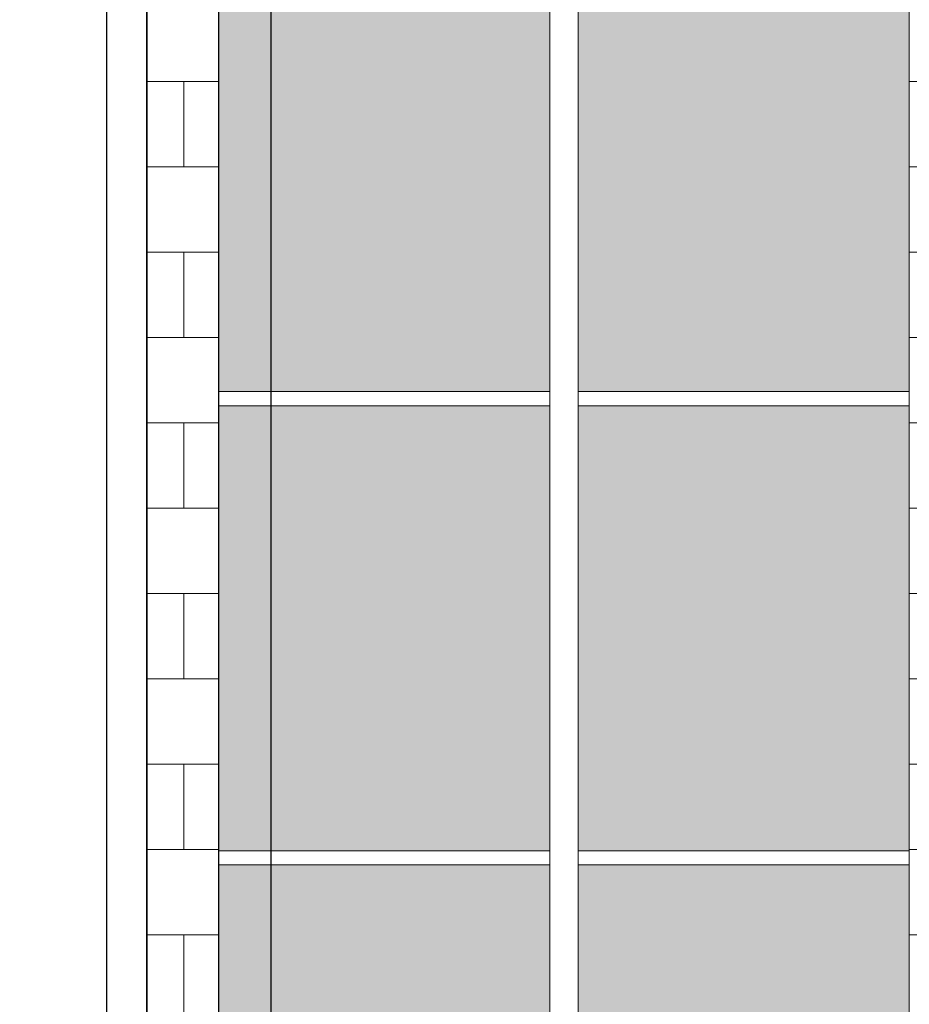
# Model space of a CAD drawing. Units: inches. Extents: x -26 to 776, y -22 to 650.
# Tile 20 of 62: x 222 to 285, y 223 to 292. Entities that reach past the tile are written whole.
import ezdxf

# ---------------------------------------------------------------- set-up
doc = ezdxf.new("R2010")
doc.units = ezdxf.units.IN
doc.header["$MEASUREMENT"] = 0
for name, color, linetype, lineweight in [('A-ANNO-DIMS', 2, 'Continuous', 18), ('A-GLAZ', 4, 'Continuous', 18), ('A-GLAZ-PATT', 9, 'Continuous', 13), ('A-WALL', 7, 'Continuous', 35), ('A-WALL-PATT', 8, 'Continuous', 13), ('A-WALL-TRIM', 7, 'Continuous', 18)]:
    doc.layers.add(name, color=color, linetype=linetype, lineweight=lineweight)
doc.styles.get("Standard").update_dxf_attribs({"font": 'arial.ttf'})
doc.dimstyles.get("Standard").update_dxf_attribs({"dimtxt": 0.5625, "dimasz": 0.18, "dimexe": 0.18, "dimexo": 0.0625, "dimgap": 0.09, "dimtad": 0, "dimtih": 1, "dimtoh": 1, "dimdec": 4, "dimzin": 0, "dimdsep": 46, "dimlunit": 4, "dimtxsty": 'Standard', "dimcen": 0.09, "dimadec": 0, "dimazin": 0, "dimtfac": 1, "dimtdec": 4, "dimtofl": 0, "dimtmove": 0, "dimatfit": 3, "dimfxl": 1, "dimtolj": 1, "dimtzin": 0, "dimarcsym": 0})

# ---------------------------------------------------------------- blocks, each defined once
blk = doc.blocks.new('WIN-ELEV-2X4-HEAD')
for p, q in [((23.276, 0), (23.276, 123)), ((25.276, 0), (25.276, 123)), ((0, 94.772), (23.276, 94.772)), ((25.276, 94.772), (48.553, 94.772)), ((0, 93.772), (23.276, 93.772)), ((25.276, 93.772), (48.553, 93.772)), ((0, 62.5), (23.276, 62.5)), ((25.276, 62.5), (48.553, 62.5)), ((0, 61.5), (23.276, 61.5)), ((25.276, 61.5), (48.553, 61.5))]:
    blk.add_line(p, q)
blk.add_lwpolyline([(48.553, 0), (0, 0), (0, 123), (48.553, 123)], close=True)
blk = doc.blocks.new('*D34')
at = {"layer": 'A-ANNO-DIMS', "color": 0, "lineweight": -2, "transparency": 16777216}
for p, q in [((228.573, 528.296), (228.573, -21.315)), ((357.303, 528.361), (357.303, -21.315)), ((228.753, -21.135), (291.707, -21.135)), ((357.123, -21.135), (294.17, -21.135))]:
    blk.add_line(p, q, dxfattribs=at)
at = {"layer": 'A-ANNO-DIMS', "color": 0, "transparency": 16777216}
for points in [[(228.753, -21.105), (228.753, -21.165), (228.573, -21.135)], [(357.123, -21.105), (357.123, -21.165), (357.303, -21.135)]]:
    blk.add_solid(points, dxfattribs=at)
at = {"layer": 'Defpoints', "color": 0, "transparency": 16777216}
for p in [(228.573, 528.358), (357.303, 528.423), (357.303, -21.135)]:
    blk.add_point(p, dxfattribs=at)
at = {"layer": 'A-ANNO-DIMS', "color": 0, "transparency": 16777216, "insert": (292.938, -21.135), "char_height": 0.5625, "attachment_point": 5}
blk.add_mtext('\\A1;128.73', dxfattribs=at)
blk = doc.blocks.new('*D43')
at = {"layer": 'A-ANNO-DIMS', "color": 0, "lineweight": -2, "transparency": 16777216}
for p, q in [((231.425, 159.545), (231.425, 649.856)), ((231.605, 649.676), (233.125, 649.676)), ((236.285, 649.676), (234.764, 649.676)), ((236.465, 171.48), (236.465, 649.856))]:
    blk.add_line(p, q, dxfattribs=at)
at = {"layer": 'A-ANNO-DIMS', "color": 0, "transparency": 16777216}
for points in [[(231.605, 649.706), (231.605, 649.646), (231.425, 649.676)], [(236.285, 649.706), (236.285, 649.646), (236.465, 649.676)]]:
    blk.add_solid(points, dxfattribs=at)
at = {"layer": 'Defpoints', "color": 0, "transparency": 16777216}
for p in [(236.465, 649.676), (236.465, 171.417), (231.425, 159.482)]:
    blk.add_point(p, dxfattribs=at)
at = {"layer": 'A-ANNO-DIMS', "color": 0, "transparency": 16777216, "insert": (233.945, 649.676), "char_height": 0.5625, "attachment_point": 5}
blk.add_mtext('\\A1;5.04', dxfattribs=at)
blk = doc.blocks.new('*D44')
at = {"layer": 'A-ANNO-DIMS', "color": 0, "lineweight": -2, "transparency": 16777216}
for p, q in [((231.425, 15.545), (231.425, 649.856)), ((231.605, 649.676), (234.975, 649.676)), ((239.985, 649.676), (236.615, 649.676)), ((240.165, 26.486), (240.165, 649.856))]:
    blk.add_line(p, q, dxfattribs=at)
at = {"layer": 'A-ANNO-DIMS', "color": 0, "transparency": 16777216}
for points in [[(231.605, 649.706), (231.605, 649.646), (231.425, 649.676)], [(239.985, 649.706), (239.985, 649.646), (240.165, 649.676)]]:
    blk.add_solid(points, dxfattribs=at)
at = {"layer": 'Defpoints', "color": 0, "transparency": 16777216}
for p in [(240.165, 649.676), (240.165, 26.424), (231.425, 15.482)]:
    blk.add_point(p, dxfattribs=at)
at = {"layer": 'A-ANNO-DIMS', "color": 0, "transparency": 16777216, "insert": (235.795, 649.676), "char_height": 0.5625, "attachment_point": 5}
blk.add_mtext('\\A1;8.74', dxfattribs=at)

msp = doc.modelspace()

# ---------------------------------------------------------------- hatches: boundary and pattern name
at = {"layer": 'A-GLAZ-PATT'}
h = msp.add_hatch(dxfattribs=at)
h.set_pattern_fill('GOST_GLASS', color=256, scale=0.75)
h.set_pattern_definition([(45, (0, 0), (6.36396, 0), [3.75, -5.25]), (45, (1.591, 0), (6.36396, 0), [1.5, -7.5]), (45, (0, 1.591), (6.36396, 0), [1.5, -7.5])])
h.paths.add_polyline_path([(115.8402, 198.8773), (93.6448, 198.8773), (93.6448, 173.9734), (115.8402, 173.9734)])
h.paths.add_polyline_path([(144.1571, 198.8773), (115.8402, 198.8773), (115.8402, 173.9734), (144.1571, 173.9734)])
h.paths.add_polyline_path([(115.8402, 224.3396), (93.6448, 224.3396), (93.6448, 198.8773), (115.8402, 198.8773)])
h.paths.add_polyline_path([(144.1571, 248.4417), (115.8402, 248.4417), (115.8402, 224.3396), (144.1571, 224.3396)])
h.paths.add_polyline_path([(144.1571, 224.3396), (115.8402, 224.3396), (115.8402, 198.8773), (144.1571, 198.8773)])
h.paths.add_polyline_path([(170.5449, 224.3396), (144.1571, 224.3396), (144.1571, 198.8773), (170.5449, 198.8773)])
h.paths.add_polyline_path([(170.5449, 198.8773), (144.1571, 198.8773), (144.1571, 173.9734), (170.5449, 173.9734)])
h.paths.add_polyline_path([(194.6694, 198.8773), (170.5449, 198.8773), (170.5449, 173.9734), (194.6694, 173.9734)])
h.paths.add_polyline_path([(194.6694, 224.3396), (170.5449, 224.3396), (170.5449, 198.8773), (194.6694, 198.8773)])
h.paths.add_polyline_path([(194.6694, 248.4417), (170.5449, 248.4417), (170.5449, 224.3396), (194.6694, 224.3396)])
h.paths.add_polyline_path([(170.5449, 248.4417), (144.1571, 248.4417), (144.1571, 224.3396), (170.5449, 224.3396)])
h.paths.add_polyline_path([(144.1571, 269.3091), (115.8402, 269.3091), (115.8402, 248.4417), (144.1571, 248.4417)])
h.paths.add_polyline_path([(115.8402, 269.3091), (93.6448, 269.3091), (93.6448, 248.4417), (115.8402, 248.4417)])
h.paths.add_polyline_path([(115.8402, 248.4417), (93.6448, 248.4417), (93.6448, 224.3396), (115.8402, 224.3396)])
h.paths.add_polyline_path([(170.5449, 269.3091), (144.1571, 269.3091), (144.1571, 248.4417), (170.5449, 248.4417)])
h.paths.add_polyline_path([(194.6694, 269.3091), (170.5449, 269.3091), (170.5449, 248.4417), (194.6694, 248.4417)])
h.paths.add_polyline_path([(259.7413, 294.4171), (236.4647, 294.4171), (236.4647, 266.1888), (259.7413, 266.1888)])
h.paths.add_polyline_path([(285.0179, 294.4171), (261.7413, 294.4171), (261.7413, 266.1888), (285.0179, 266.1888)])
h.paths.add_polyline_path([(285.0179, 265.1888), (261.7413, 265.1888), (261.7413, 233.9172), (285.0179, 233.9172)])
h.paths.add_polyline_path([(259.7413, 265.1888), (236.4647, 265.1888), (236.4647, 233.9172), (259.7413, 233.9172)])
h.paths.add_polyline_path([(259.7413, 232.9172), (236.4647, 232.9172), (236.4647, 207.1741), (259.7413, 207.1741)])
h.paths.add_polyline_path([(285.0179, 232.9172), (261.7413, 232.9172), (261.7413, 207.1741), (285.0179, 207.1741)])
h.paths.add_polyline_path([(285.0179, 206.1741), (261.7413, 206.1741), (261.7413, 199.3298), (278.1134, 199.3298), (278.1134, 171.4173), (285.0179, 171.4173)])
h.paths.add_polyline_path([(259.7413, 206.1741), (236.4647, 206.1741), (236.4647, 199.3298), (259.7413, 199.3298)])
h.paths.add_polyline_path([(259.7413, 197.3298), (236.4647, 197.3298), (236.4647, 171.4173), (259.7413, 171.4173)])
h.paths.add_polyline_path([(276.1134, 197.3298), (261.7413, 197.3298), (261.7413, 171.4173), (276.1134, 171.4173)], flags=17)
h.paths.add_polyline_path([(255.8125, 548.0348), (228.5733, 548.0348), (228.5733, 528.3585), (255.8125, 528.3585)])
h.paths.add_polyline_path([(281.6181, 548.0348), (256.0792, 548.0348), (256.0792, 528.3585), (281.6181, 528.3585)])
h.paths.add_polyline_path([(308.8797, 548.0348), (281.789, 548.0348), (281.789, 528.3585), (308.8797, 528.3585)])
h.paths.add_polyline_path([(357.2724, 548.0995), (309.2457, 548.0348), (309.2457, 528.3585), (357.3034, 528.4233), (357.3034, 538.2614)])
h.paths.add_polyline_path([(259.7413, 437.1188), (236.4647, 437.1188), (236.4647, 408.8905), (259.7413, 408.8905)])
h.paths.add_polyline_path([(285.0179, 437.1188), (261.7413, 437.1188), (261.7413, 408.8905), (285.0179, 408.8905)])
h.paths.add_polyline_path([(259.7413, 407.8905), (236.4647, 407.8905), (236.4647, 376.6189), (259.7413, 376.6189)])
h.paths.add_polyline_path([(285.0179, 407.8905), (261.7413, 407.8905), (261.7413, 376.6189), (285.0179, 376.6189)])
h.paths.add_polyline_path([(285.0179, 375.6189), (261.7413, 375.6189), (261.7413, 349.8758), (285.0179, 349.8758)])
h.paths.add_polyline_path([(285.0179, 348.8758), (261.7413, 348.8758), (261.7413, 314.119), (285.0179, 314.119)])
h.paths.add_polyline_path([(259.7413, 348.8758), (236.4647, 348.8758), (236.4647, 314.119), (259.7413, 314.119)])
h.paths.add_polyline_path([(259.7413, 375.6189), (236.4647, 375.6189), (236.4647, 349.8758), (259.7413, 349.8758)])
h.paths.add_polyline_path([(194.6694, 404.1909), (170.5449, 404.1909), (170.5449, 383.3235), (194.6694, 383.3235)])
h.paths.add_polyline_path([(170.5449, 404.1909), (144.1571, 404.1909), (144.1571, 383.3235), (170.5449, 383.3235)])
h.paths.add_polyline_path([(144.1571, 404.1909), (115.8402, 404.1909), (115.8402, 383.3235), (144.1571, 383.3235)])
h.paths.add_polyline_path([(115.8402, 404.1909), (93.6448, 404.1909), (93.6448, 383.3235), (115.8402, 383.3235)])
h.paths.add_polyline_path([(115.8402, 383.3235), (93.6448, 383.3235), (93.6448, 359.2214), (115.8402, 359.2214)])
h.paths.add_polyline_path([(144.1571, 383.3235), (115.8402, 383.3235), (115.8402, 359.2214), (144.1571, 359.2214)])
h.paths.add_polyline_path([(115.8402, 359.2214), (93.6448, 359.2214), (93.6448, 333.7591), (115.8402, 333.7591)])
h.paths.add_polyline_path([(144.1571, 359.2214), (115.8402, 359.2214), (115.8402, 333.7591), (144.1571, 333.7591)])
h.paths.add_polyline_path([(115.8402, 333.7591), (93.6448, 333.7591), (93.6448, 308.8552), (115.8402, 308.8552)])
h.paths.add_polyline_path([(144.1571, 333.7591), (115.8402, 333.7591), (115.8402, 308.8552), (144.1571, 308.8552)])
h.paths.add_polyline_path([(170.5449, 333.7591), (144.1571, 333.7591), (144.1571, 308.8552), (170.5449, 308.8552)])
h.paths.add_polyline_path([(170.5449, 359.2214), (144.1571, 359.2214), (144.1571, 333.7591), (170.5449, 333.7591)])
h.paths.add_polyline_path([(170.5449, 383.3235), (144.1571, 383.3235), (144.1571, 359.2214), (170.5449, 359.2214)])
h.paths.add_polyline_path([(194.6694, 383.3235), (170.5449, 383.3235), (170.5449, 359.2214), (194.6694, 359.2214)])
h.paths.add_polyline_path([(194.6694, 359.2214), (170.5449, 359.2214), (170.5449, 333.7591), (194.6694, 333.7591)])
h.paths.add_polyline_path([(194.6694, 333.7591), (170.5449, 333.7591), (170.5449, 308.8552), (194.6694, 308.8552)])
at = {"layer": 'A-WALL-PATT'}
h = msp.add_hatch(dxfattribs=at)
h.set_pattern_fill('AR-B816', color=256, scale=0.75)
h.paths.add_polyline_path([(289.2424, 504.4205), (231.4249, 504.4205), (231.4249, 458.1203), (231.4249, 221.6413), (231.4249, 209.6413), (231.4249, 159.4824), (285.0179, 159.4824), (285.0179, 171.4173), (236.4647, 171.4173), (236.4647, 294.4171), (236.4647, 303.3046), (285.0179, 303.3046), (285.0179, 294.4171), (285.0179, 171.4173), (285.0179, 159.4824), (289.2424, 159.4824), (289.2424, 291.1798), (289.2424, 458.1203)])
h.paths.add_polyline_path([(285.0179, 446.0063), (285.0179, 437.1188), (285.0179, 314.119), (236.4647, 314.119), (236.4647, 437.1188), (236.4647, 446.0063)], flags=16)

# ---------------------------------------------------------------- linework, layer by layer
at = {"layer": 'A-WALL'}
msp.add_line((231.4249, 221.6413), (231.4249, 458.1203), dxfattribs=at)
at = {"layer": 'A-WALL-TRIM'}
msp.add_line((285.0179, 15.4824), (285.0179, 249.6598), dxfattribs=at)

# ---------------------------------------------------------------- block references
at = {"layer": 'A-GLAZ'}
msp.add_blockref('WIN-ELEV-2X4-HEAD', (236.465, 171.417), dxfattribs=at)

# ---------------------------------------------------------------- dimensions: what is measured, and where the dimension line sits
at = {"layer": 'A-ANNO-DIMS'}
for base, p1, p2, picture, middle in [((236.4647, 649.6763), (231.4249, 159.4824), (236.4647, 171.4173), '*D43', (233.9448, 649.6763)), ((240.1654, 649.6763), (231.4249, 15.4824), (240.1654, 26.4239), '*D44', (235.7952, 649.6763)), ((357.3034, -21.1349), (228.5733, 528.3585), (357.3034, 528.4233), '*D34', (292.9384, -21.1349))]:
    dim = msp.add_linear_dim(base=base, p1=p1, p2=p2, dimstyle='Standard', override={"dimdec": 2, "dimlfac": 1, "dimrnd": 0, "dimzin": 0, "dimdsep": 46, "dimlunit": 2}, dxfattribs=at)
    dim.commit()
    dim.dimension.update_dxf_attribs({"geometry": picture, "text_midpoint": middle})

doc.saveas('drawing.dxf')
